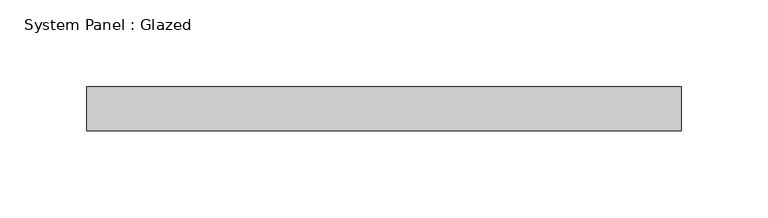
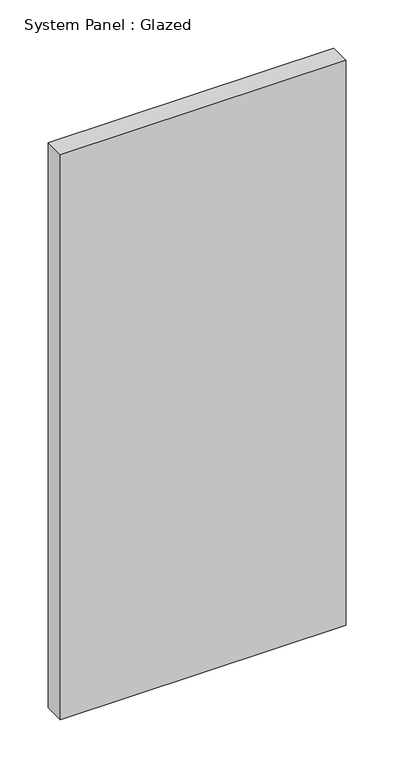
"""IFC4 building model written with IfcOpenShell, lengths in millimetres: plate geometry, System Panel : Glazed."""

from ifc_helpers import new_model, si_unit, origin, origin_with_axes, place, context, project, spatial, polyline, outline, extrude, source, transform, mapped, element, save


def system_panel_glazed_ea4b41a2(model_context):
    return source(origin(), model_context, "Body", "SweptSolid", [
        extrude(outline(polyline([(171.45, 19.05), (-171.45, 19.05), (-171.45, 44.45), (171.45, 44.45), (171.45, 19.05)])), origin_with_axes(), (0.0, 0.0, 1.0), 717.55),
    ])


if __name__ == "__main__":
    model = new_model("IFC4")
    model_context = context("Model", 3, world=origin())
    ifc_project = project(units=[si_unit("LENGTHUNIT", "METRE", prefix="MILLI")], contexts=[model_context])
    site = spatial("IfcSite", under=ifc_project)
    building = spatial("IfcBuilding", under=site)
    placement = place(None, origin())
    system_panel_glazed_shape = system_panel_glazed_ea4b41a2(model_context)
    element("IfcPlate", 1, ObjectType="System Panel : Glazed", at=placement, inside=building, context=model_context, shape_type="MappedRepresentation", body=[
        mapped(system_panel_glazed_shape, transform((0.0, 0.0, 0.0), x_axis=(1.0, 0.0, 0.0), y_axis=(0.0, 1.0, 0.0), z_axis=(0.0, 0.0, 1.0))),
    ])
    save(model, "model.ifc")

# Revit data of these elements
# Type "System Panel : Glazed"
#   Construction Type Id = "GSP4R"
#   Analytic Construction = "1/8 in Pilkington single glazing"
#   Visual Light Transmittance = 0.9
#   Solar Heat Gain Coefficient = 0.86
#   Heat Transfer Coefficient (U) = 1.18115 BTU/(h·ft²·°F)
# Element 1 (IfcPlate, "System Panel : Glazed")
#   Materials on its faces: "Glass"
# Materials
#   "Glass": class "Glass", colour RGB 0 128 192, transparency 0.75, Description = "Soda Lime Glass", Cost = 0
